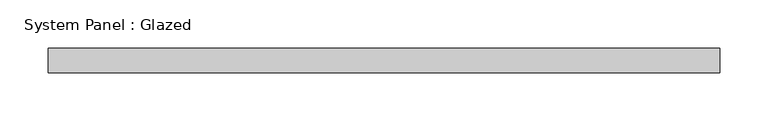
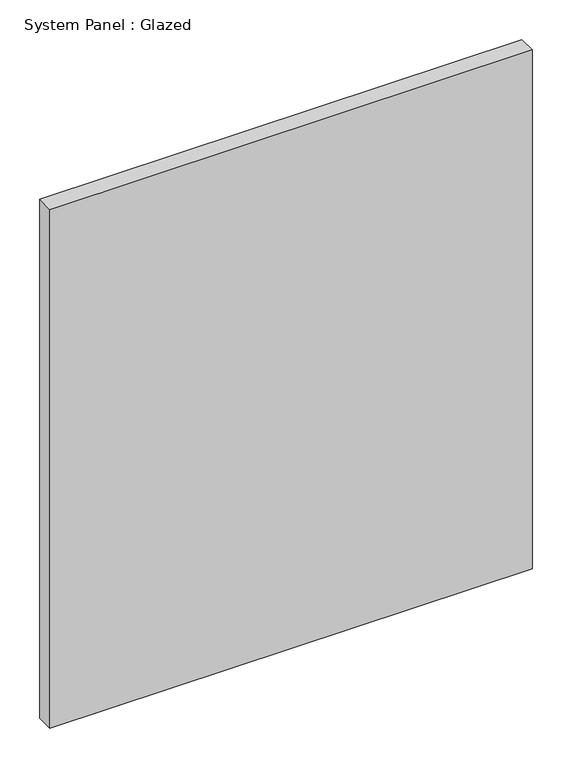
"""IFC4 building model written with IfcOpenShell, lengths in millimetres: plate geometry, System Panel : Glazed."""

from ifc_helpers import new_model, si_unit, origin, origin_with_axes, place, context, project, spatial, polyline, outline, extrude, source, transform, mapped, element, save


def system_panel_glazed_55fd798e(model_context):
    return source(origin(), model_context, "Body", "SweptSolid", [
        extrude(outline(polyline([(349.25, 19.05), (-349.25, 19.05), (-349.25, 44.45), (349.25, 44.45), (349.25, 19.05)])), origin_with_axes(), (0.0, 0.0, 1.0), 794.4489237),
    ])


if __name__ == "__main__":
    model = new_model("IFC4")
    model_context = context("Model", 3, world=origin())
    ifc_project = project(units=[si_unit("LENGTHUNIT", "METRE", prefix="MILLI")], contexts=[model_context])
    site = spatial("IfcSite", under=ifc_project)
    building = spatial("IfcBuilding", under=site)
    placement = place(None, origin())
    system_panel_glazed_shape = system_panel_glazed_55fd798e(model_context)
    element("IfcPlate", 1, ObjectType="System Panel : Glazed", at=placement, inside=building, context=model_context, shape_type="MappedRepresentation", body=[
        mapped(system_panel_glazed_shape, transform((0.0, 0.0, 0.0), x_axis=(1.0, 0.0, 0.0), y_axis=(0.0, 1.0, 0.0), z_axis=(0.0, 0.0, 1.0))),
    ])
    save(model, "model.ifc")

# Revit data of these elements
# Type "System Panel : Glazed"
#   Construction Type Id = "GSP4R"
#   Analytic Construction = "1/8 in Pilkington single glazing"
#   Visual Light Transmittance = 0.9
#   Solar Heat Gain Coefficient = 0.86
#   Heat Transfer Coefficient (U) = 1.18115 BTU/(h·ft²·°F)
#   Define Thermal Properties by = 1
# Element 1 (IfcPlate, "System Panel : Glazed")
#   Materials on its faces: "Glass"
# Materials
#   "Glass": class "Glass", colour RGB 0 128 192, transparency 0.75, Description = "Soda Lime Glass", Cost = 0
